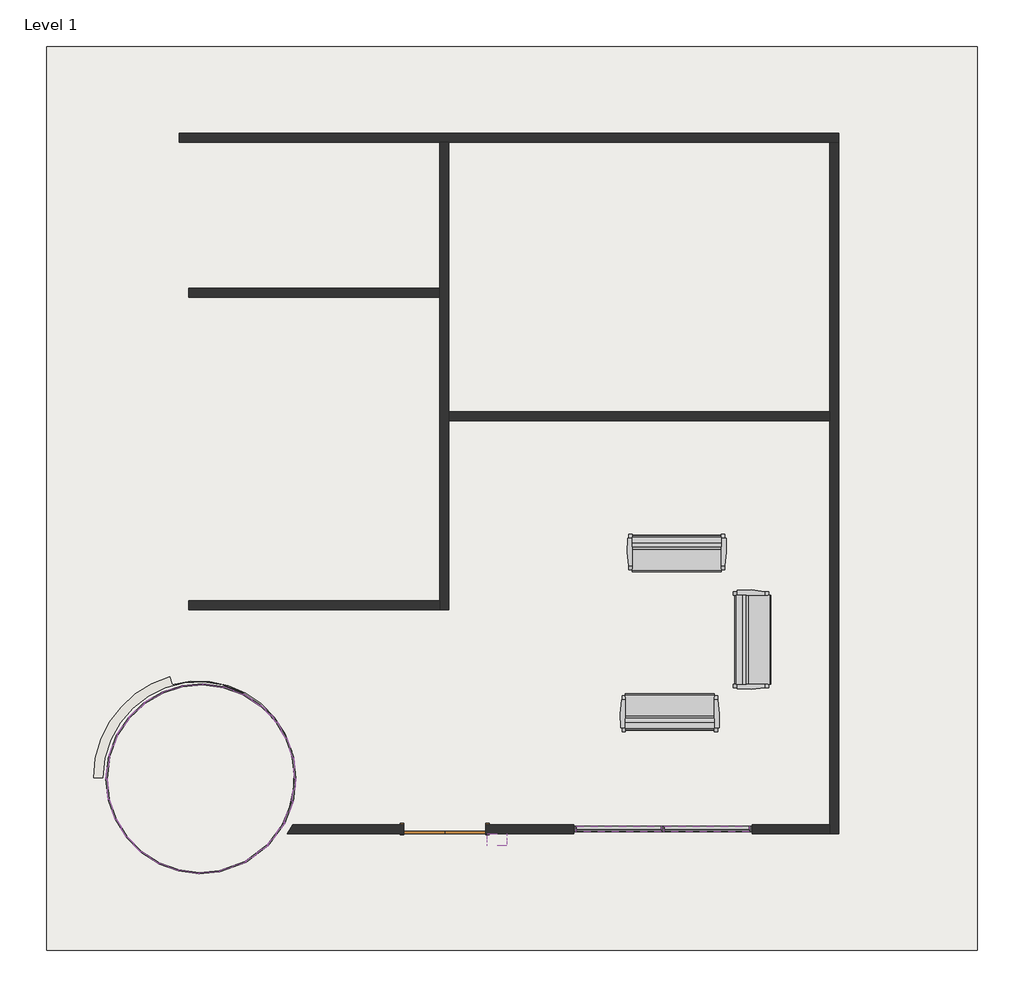
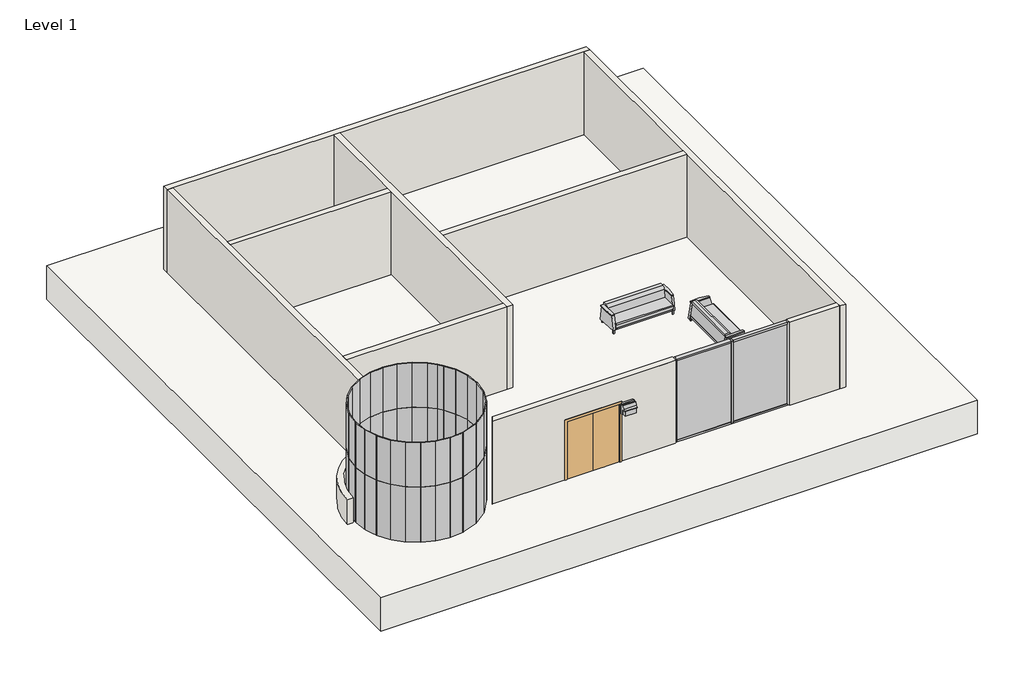
# One storey, incomplete: 58 plates, 11 walls, 7 members, 3 furniture elements, 1 door, 1 light fixture, 1 slab.
"""IFC4 building model written with IfcOpenShell, lengths in millimetres."""

from ifc_helpers import new_model, si_unit, point, frame, frame_2d, origin, origin_with_axes, place, context, project, spatial, polyline, circle_curve, trimmed, segment, composite_curve, outline, extrude, faceted_brep, transform, mapped, element, save
from ifc_brep_helpers import plane_surface, revolved_surface, advanced_brep
from components import door_0b985982, furniture_aff9b2fb, wall_pack_light_exterior_120v_50d39a1a, member_eaba9652, member_3f395ae9, member_7b893d20, system_panel_glazed_c6a8e7fc, system_panel_glazed_f1c144f9, system_panel_glazed_8ed2b2ee, system_panel_glazed_c7815b78, system_panel_glazed_220ba5f3, system_panel_glazed_11fb153e, system_panel_glazed_2f540b85, system_panel_glazed_4848e608, system_panel_glazed_8b35a0ff, system_panel_glazed_87282c25, system_panel_glazed_6d1bb68c, system_panel_glazed_cb3ffd69, system_panel_glazed_404d015f

model = new_model("IFC4")

# Units and contexts
model_context = context("Model", 3, world=origin())
ifc_project = project(units=[si_unit("LENGTHUNIT", "METRE", prefix="MILLI")], contexts=[model_context])

# Site, building, storey
site = spatial("IfcSite", under=ifc_project)
building = spatial("IfcBuilding", under=site)
storey = spatial("IfcBuildingStorey", under=building, Name="Level 1", Elevation=0.0)

# Door
placement = place(None, origin())
door_shape = door_0b985982(model_context)
element("IfcDoor", 1, ObjectType="Door-Double-Flush_Panel : 72\" x 84\"", at=placement, inside=storey, context=model_context, shape_type="MappedRepresentation", body=[
    mapped(door_shape, transform((-7135.1683746, -2219.4937024, 0.0), x_axis=(-1.0, 0.0, 0.0), y_axis=(0.0, -1.0, 0.0), z_axis=(0.0, 0.0, 1.0))),
])

# Furniture
furniture_shape = furniture_aff9b2fb(model_context)
element("IfcFurniture", 2, ObjectType="Sofa-Pensi : 84\"", at=placement, inside=storey, context=model_context, shape_type="MappedRepresentation", body=[
    mapped(furniture_shape, transform((-2244.8524991, 3650.1964615, 0.0), x_axis=(1.0, 0.0, 0.0), y_axis=(0.0, 1.0, 0.0), z_axis=(0.0, 0.0, 1.0))),
])
element("IfcFurniture", 3, ObjectType="Sofa-Pensi : 84\"", at=placement, inside=storey, context=model_context, shape_type="MappedRepresentation", body=[
    mapped(furniture_shape, transform((-12.736413, 1720.492712, 0.0), x_axis=(0.0, 1.0000000000000002, 0.0), y_axis=(-1.0000000000000002, 0.0, 0.0), z_axis=(0.0, 0.0, 1.0))),
])
element("IfcFurniture", 4, ObjectType="Sofa-Pensi : 84\"", at=placement, inside=storey, context=model_context, shape_type="MappedRepresentation", body=[
    mapped(furniture_shape, transform((-1840.0399991, 648.4161336, 0.0), x_axis=(-1.0000000000000004, 0.0, 0.0), y_axis=(0.0, -1.0000000000000004, 0.0), z_axis=(0.0, 0.0, 1.0))),
])

# Light fixture
wall_pack_light_exterior_120v_shape = wall_pack_light_exterior_120v_50d39a1a(model_context)
element("IfcLightFixture", 5, ObjectType="Wall Pack Light - Exterior : 120V", at=placement, inside=storey, context=model_context, shape_type="MappedRepresentation", body=[
    mapped(wall_pack_light_exterior_120v_shape, transform((-5845.0043181, -2219.4937024, -589.106918), x_axis=(-1.0, 0.0, 0.0), y_axis=(0.0, -1.0, 0.0), z_axis=(0.0, 0.0, 1.0))),
])

# Members
member_shape = member_eaba9652(model_context)
element("IfcMember", 6, ObjectType="Rectangular Mullion : 2.5\" x 5\" rectangular", at=placement, inside=storey, context=model_context, shape_type="MappedRepresentation", body=[
    mapped(member_shape, transform((-2277.4073118, -2219.4937024, 0.0), x_axis=(-1.0, 0.0, 0.0), y_axis=(0.0, 1.0, 0.0), z_axis=(0.0, 0.0, -1.0))),
])
member_2_shape = member_3f395ae9(model_context)
element("IfcMember", 7, ObjectType="Rectangular Mullion : 2.5\" x 5\" rectangular", at=placement, inside=storey, context=model_context, shape_type="MappedRepresentation", body=[
    mapped(member_2_shape, transform((-4264.9683746, -2219.4937024, 0.0), x_axis=(-1.0, 0.0, 0.0), y_axis=(0.0, 1.0, 0.0), z_axis=(0.0, 0.0, -1.0))),
])
element("IfcMember", 8, ObjectType="Rectangular Mullion : 2.5\" x 5\" rectangular", at=placement, inside=storey, context=model_context, shape_type="MappedRepresentation", body=[
    mapped(member_2_shape, transform((-289.8462491, -2219.4937024, 3048.0), x_axis=(1.0, 0.0, 0.0), y_axis=(0.0, 1.0, 0.0), z_axis=(0.0, 0.0, 1.0))),
])
member_3_shape = member_7b893d20(model_context)
element("IfcMember", 9, ObjectType="Rectangular Mullion : 2.5\" x 5\" rectangular", at=placement, inside=storey, context=model_context, shape_type="MappedRepresentation", body=[
    mapped(member_3_shape, transform((-4201.4683746, -2219.4937024, 3048.0), x_axis=(0.0, 0.0, 1.0), y_axis=(0.0, 1.0, 0.0), z_axis=(-1.0, 0.0, 0.0))),
])
element("IfcMember", 10, ObjectType="Rectangular Mullion : 2.5\" x 5\" rectangular", at=placement, inside=storey, context=model_context, shape_type="MappedRepresentation", body=[
    mapped(member_3_shape, transform((-2245.6573118, -2219.4937024, 3048.0), x_axis=(0.0, 0.0, 1.0), y_axis=(0.0, 1.0, 0.0), z_axis=(-1.0, 0.0, 0.0))),
])
element("IfcMember", 11, ObjectType="Rectangular Mullion : 2.5\" x 5\" rectangular", at=placement, inside=storey, context=model_context, shape_type="MappedRepresentation", body=[
    mapped(member_3_shape, transform((-353.3462491, -2219.4937024, 0.0), x_axis=(0.0, 0.0, -1.0), y_axis=(0.0, 1.0, 0.0), z_axis=(1.0, 0.0, 0.0))),
])
element("IfcMember", 12, ObjectType="Rectangular Mullion : 2.5\" x 5\" rectangular", at=placement, inside=storey, context=model_context, shape_type="MappedRepresentation", body=[
    mapped(member_3_shape, transform((-2309.1573118, -2219.4937024, 0.0), x_axis=(0.0, 0.0, -1.0), y_axis=(0.0, 1.0, 0.0), z_axis=(1.0, 0.0, 0.0))),
])

# Plates
system_panel_glazed_shape = system_panel_glazed_c6a8e7fc(model_context)
element("IfcPlate", 13, ObjectType="System Panel : Glazed", at=placement, inside=storey, context=model_context, shape_type="MappedRepresentation", body=[
    mapped(system_panel_glazed_shape, transform((-1299.5017804, -2219.4937024, 63.5), x_axis=(-1.0, 0.0, 0.0), y_axis=(0.0, -1.0, 0.0), z_axis=(0.0, 0.0, 1.0))),
])
element("IfcPlate", 14, ObjectType="System Panel : Glazed", at=placement, inside=storey, context=model_context, shape_type="MappedRepresentation", body=[
    mapped(system_panel_glazed_shape, transform((-3255.3128432, -2219.4937024, 63.5), x_axis=(-1.0, 0.0, 0.0), y_axis=(0.0, -1.0, 0.0), z_axis=(0.0, 0.0, 1.0))),
])
system_panel_glazed_2_shape = system_panel_glazed_f1c144f9(model_context)
element("IfcPlate", 15, ObjectType="System Panel : Glazed", at=placement, inside=storey, context=model_context, shape_type="MappedRepresentation", body=[
    mapped(system_panel_glazed_2_shape, transform((-14541.9245022, -346.5978939, 0.0), x_axis=(-0.3551689475306269, -0.9348021281051873, 0.0), y_axis=(0.9348021281051873, -0.3551689475306269, 0.0), z_axis=(0.0, 0.0, 1.0))),
])
element("IfcPlate", 16, ObjectType="System Panel : Glazed", at=placement, inside=storey, context=model_context, shape_type="MappedRepresentation", body=[
    mapped(system_panel_glazed_2_shape, transform((-10582.1178502, -1851.0877948, 0.0), x_axis=(0.35516894753064066, 0.934802128105182, 0.0), y_axis=(-0.934802128105182, 0.35516894753064066, 0.0), z_axis=(0.0, 0.0, 1.0))),
])
element("IfcPlate", 17, ObjectType="System Panel : Glazed", at=placement, inside=storey, context=model_context, shape_type="MappedRepresentation", body=[
    mapped(system_panel_glazed_2_shape, transform((-10459.5232171, -1354.5613954, 0.0), x_axis=(0.12073632210407238, 0.9926846128175765, 0.0), y_axis=(-0.9926846128175765, 0.12073632210407238, 0.0), z_axis=(0.0, 0.0, 1.0))),
])
element("IfcPlate", 18, ObjectType="System Panel : Glazed", at=placement, inside=storey, context=model_context, shape_type="MappedRepresentation", body=[
    mapped(system_panel_glazed_2_shape, transform((-14664.5191354, -843.1242933, 0.0), x_axis=(-0.12073632210406242, -0.9926846128175777, 0.0), y_axis=(0.9926846128175777, -0.12073632210406242, 0.0), z_axis=(0.0, 0.0, 1.0))),
])
system_panel_glazed_3_shape = system_panel_glazed_8ed2b2ee(model_context)
element("IfcPlate", 19, ObjectType="System Panel : Glazed", at=placement, inside=storey, context=model_context, shape_type="MappedRepresentation", body=[
    mapped(system_panel_glazed_3_shape, transform((-11841.3777431, -3082.3793017, 0.0), x_axis=(0.9398911711666007, 0.34147413718036645, 0.0), y_axis=(-0.34147413718036645, 0.9398911711666007, 0.0), z_axis=(0.0, 0.0, 1.0))),
])
element("IfcPlate", 20, ObjectType="System Panel : Glazed", at=placement, inside=storey, context=model_context, shape_type="MappedRepresentation", body=[
    mapped(system_panel_glazed_3_shape, transform((-10858.9635423, -2345.1728692, 0.0), x_axis=(0.5905687200141164, 0.8069873524045393, 0.0), y_axis=(-0.8069873524045393, 0.5905687200141164, 0.0), z_axis=(0.0, 0.0, 1.0))),
])
element("IfcPlate", 21, ObjectType="System Panel : Glazed", at=placement, inside=storey, context=model_context, shape_type="MappedRepresentation", body=[
    mapped(system_panel_glazed_3_shape, transform((-11295.3522982, -2786.8279712, 0.0), x_axis=(0.7998453025525061, 0.6002062078858317, 0.0), y_axis=(-0.6002062078858317, 0.7998453025525061, 0.0), z_axis=(0.0, 0.0, 1.0))),
])
system_panel_glazed_4_shape = system_panel_glazed_c7815b78(model_context)
element("IfcPlate", 22, ObjectType="System Panel : Glazed", at=placement, inside=storey, context=model_context, shape_type="MappedRepresentation", body=[
    mapped(system_panel_glazed_4_shape, transform((-10454.4737362, -864.5204039, 0.0), x_axis=(-0.11050163420416613, 0.993875942378227, 0.0), y_axis=(-0.993875942378227, -0.11050163420416613, 0.0), z_axis=(0.0, 0.0, 1.0))),
])
element("IfcPlate", 23, ObjectType="System Panel : Glazed", at=placement, inside=storey, context=model_context, shape_type="MappedRepresentation", body=[
    mapped(system_panel_glazed_4_shape, transform((-14669.5686163, -1333.1652848, 0.0), x_axis=(0.11050163420415138, -0.9938759423782286, 0.0), y_axis=(0.9938759423782286, 0.11050163420415138, 0.0), z_axis=(0.0, 0.0, 1.0))),
])
element("IfcPlate", 24, ObjectType="System Panel : Glazed", at=placement, inside=storey, context=model_context, shape_type="MappedRepresentation", body=[
    mapped(system_panel_glazed_4_shape, transform((-11410.1424167, 681.5611944, 0.0), x_axis=(-0.8396018558176894, 0.5432022861766066, 0.0), y_axis=(-0.5432022861766066, -0.8396018558176894, 0.0), z_axis=(0.0, 0.0, 1.0))),
])
element("IfcPlate", 25, ObjectType="System Panel : Glazed", at=placement, inside=storey, context=model_context, shape_type="MappedRepresentation", body=[
    mapped(system_panel_glazed_4_shape, transform((-13212.0893695, 919.590846, 0.0), x_axis=(-0.9518517343814786, -0.3065587639506839, 0.0), y_axis=(0.3065587639506839, -0.9518517343814786, 0.0), z_axis=(0.0, 0.0, 1.0))),
])
element("IfcPlate", 26, ObjectType="System Panel : Glazed", at=placement, inside=storey, context=model_context, shape_type="MappedRepresentation", body=[
    mapped(system_panel_glazed_4_shape, transform((-12839.7224363, -3201.1142893, 0.0), x_axis=(0.9913878918151698, -0.1309581916577702, 0.0), y_axis=(0.1309581916577702, 0.9913878918151698, 0.0), z_axis=(0.0, 0.0, 1.0))),
])
element("IfcPlate", 27, ObjectType="System Panel : Glazed", at=placement, inside=storey, context=model_context, shape_type="MappedRepresentation", body=[
    mapped(system_panel_glazed_4_shape, transform((-14365.783041, -2213.7896382, 0.0), x_axis=(0.5257859322352114, -0.8506169252157811, 0.0), y_axis=(0.8506169252157811, 0.5257859322352114, 0.0), z_axis=(0.0, 0.0, 1.0))),
])
element("IfcPlate", 28, ObjectType="System Panel : Glazed", at=placement, inside=storey, context=model_context, shape_type="MappedRepresentation", body=[
    mapped(system_panel_glazed_4_shape, transform((-13713.8999358, -2879.2468831, 0.0), x_axis=(0.8396018558176805, -0.5432022861766201, 0.0), y_axis=(0.5432022861766201, 0.8396018558176805, 0.0), z_axis=(0.0, 0.0, 1.0))),
])
element("IfcPlate", 29, ObjectType="System Panel : Glazed", at=placement, inside=storey, context=model_context, shape_type="MappedRepresentation", body=[
    mapped(system_panel_glazed_4_shape, transform((-14014.4059364, 446.2272921, 0.0), x_axis=(-0.7286232370002992, -0.6849147235263715, 0.0), y_axis=(0.6849147235263715, -0.7286232370002992, 0.0), z_axis=(0.0, 0.0, 1.0))),
])
element("IfcPlate", 30, ObjectType="System Panel : Glazed", at=placement, inside=storey, context=model_context, shape_type="MappedRepresentation", body=[
    mapped(system_panel_glazed_4_shape, transform((-12284.3199161, 1003.4286006, 0.0), x_axis=(-0.9913878918151723, 0.1309581916577514, 0.0), y_axis=(-0.1309581916577514, -0.9913878918151723, 0.0), z_axis=(0.0, 0.0, 1.0))),
])
element("IfcPlate", 31, ObjectType="System Panel : Glazed", at=placement, inside=storey, context=model_context, shape_type="MappedRepresentation", body=[
    mapped(system_panel_glazed_4_shape, transform((-12752.8652893, 1013.0855973, 0.0), x_axis=(-0.9959419324521102, -0.08999815100076568, 0.0), y_axis=(0.08999815100076568, -0.9959419324521102, 0.0), z_axis=(0.0, 0.0, 1.0))),
])
element("IfcPlate", 32, ObjectType="System Panel : Glazed", at=placement, inside=storey, context=model_context, shape_type="MappedRepresentation", body=[
    mapped(system_panel_glazed_4_shape, transform((-11829.3381514, 891.0915272, 0.0), x_axis=(-0.9384120429483949, 0.34551821608913763, 0.0), y_axis=(-0.34551821608913763, -0.9384120429483949, 0.0), z_axis=(0.0, 0.0, 1.0))),
])
element("IfcPlate", 33, ObjectType="System Panel : Glazed", at=placement, inside=storey, context=model_context, shape_type="MappedRepresentation", body=[
    mapped(system_panel_glazed_4_shape, transform((-10557.4115054, -407.3204039, 0.0), x_axis=(-0.3261077326604367, 0.9453326116764772, 0.0), y_axis=(-0.9453326116764772, -0.3261077326604367, 0.0), z_axis=(0.0, 0.0, 1.0))),
])
element("IfcPlate", 34, ObjectType="System Panel : Glazed", at=placement, inside=storey, context=model_context, shape_type="MappedRepresentation", body=[
    mapped(system_panel_glazed_4_shape, transform((-12371.1770631, -3210.771286, 0.0), x_axis=(0.9959419324521115, 0.08999815100075, 0.0), y_axis=(-0.08999815100075, 0.9959419324521115, 0.0), z_axis=(0.0, 0.0, 1.0))),
])
element("IfcPlate", 35, ObjectType="System Panel : Glazed", at=placement, inside=storey, context=model_context, shape_type="MappedRepresentation", body=[
    mapped(system_panel_glazed_4_shape, transform((-13294.7042011, -3088.7772159, 0.0), x_axis=(0.9384120429483891, -0.34551821608915334, 0.0), y_axis=(0.34551821608915334, 0.9384120429483891, 0.0), z_axis=(0.0, 0.0, 1.0))),
])
element("IfcPlate", 36, ObjectType="System Panel : Glazed", at=placement, inside=storey, context=model_context, shape_type="MappedRepresentation", body=[
    mapped(system_panel_glazed_4_shape, transform((-14076.8350959, -2582.7572647, 0.0), x_axis=(0.6997834615185511, -0.7143550286692988, 0.0), y_axis=(0.7143550286692988, 0.6997834615185511, 0.0), z_axis=(0.0, 0.0, 1.0))),
])
element("IfcPlate", 37, ObjectType="System Panel : Glazed", at=placement, inside=storey, context=model_context, shape_type="MappedRepresentation", body=[
    mapped(system_panel_glazed_4_shape, transform((-14566.6308471, -1790.3652848, 0.0), x_axis=(0.32610773266042153, -0.9453326116764824, 0.0), y_axis=(0.9453326116764824, 0.32610773266042153, 0.0), z_axis=(0.0, 0.0, 1.0))),
])
element("IfcPlate", 38, ObjectType="System Panel : Glazed", at=placement, inside=storey, context=model_context, shape_type="MappedRepresentation", body=[
    mapped(system_panel_glazed_4_shape, transform((-14318.3113206, 89.4787227, 0.0), x_axis=(-0.5603879632167612, -0.8282302401396425, 0.0), y_axis=(0.8282302401396425, -0.5603879632167612, 0.0), z_axis=(0.0, 0.0, 1.0))),
])
element("IfcPlate", 39, ObjectType="System Panel : Glazed", at=placement, inside=storey, context=model_context, shape_type="MappedRepresentation", body=[
    mapped(system_panel_glazed_4_shape, transform((-13639.5625299, 727.5108588, 0.0), x_axis=(-0.8612707706620223, -0.508146297441245, 0.0), y_axis=(0.508146297441245, -0.8612707706620223, 0.0), z_axis=(0.0, 0.0, 1.0))),
])
system_panel_glazed_5_shape = system_panel_glazed_220ba5f3(model_context)
element("IfcPlate", 40, ObjectType="System Panel : Glazed", at=placement, inside=storey, context=model_context, shape_type="MappedRepresentation", body=[
    mapped(system_panel_glazed_5_shape, transform((-10742.3305673, -4.7597883, 0.0), x_axis=(-0.5152811917631037, 0.8570211744263939, 0.0), y_axis=(-0.8570211744263939, -0.5152811917631037, 0.0), z_axis=(0.0, 0.0, 1.0))),
])
system_panel_glazed_6_shape = system_panel_glazed_11fb153e(model_context)
element("IfcPlate", 41, ObjectType="System Panel : Glazed", at=placement, inside=storey, context=model_context, shape_type="MappedRepresentation", body=[
    mapped(system_panel_glazed_6_shape, transform((-11098.0043985, 445.2241463, 0.0), x_axis=(-0.7256671855033587, 0.6880458821064435, 0.0), y_axis=(-0.6880458821064435, -0.7256671855033587, 0.0), z_axis=(0.0, 0.0, 1.0))),
])
system_panel_glazed_7_shape = system_panel_glazed_2f540b85(model_context)
element("IfcPlate", 42, ObjectType="System Panel : Glazed", at=placement, inside=storey, context=model_context, shape_type="MappedRepresentation", body=[
    mapped(system_panel_glazed_7_shape, transform((-10917.0903061, 255.9395759, 0.0), x_axis=(-0.6357445726375757, 0.7718995001694627, 0.0), y_axis=(-0.7718995001694627, -0.6357445726375757, 0.0), z_axis=(0.0, 0.0, 1.0))),
])
system_panel_glazed_8_shape = system_panel_glazed_4848e608(model_context)
element("IfcPlate", 43, ObjectType="System Panel : Glazed", at=placement, inside=storey, context=model_context, shape_type="MappedRepresentation", body=[
    mapped(system_panel_glazed_8_shape, transform((-14669.5686163, -1333.1652848, 2032.0), x_axis=(0.11050163420415136, -0.9938759423782286, 0.0), y_axis=(0.9938759423782286, 0.11050163420415136, 0.0), z_axis=(0.0, 0.0, 1.0))),
])
element("IfcPlate", 44, ObjectType="System Panel : Glazed", at=placement, inside=storey, context=model_context, shape_type="MappedRepresentation", body=[
    mapped(system_panel_glazed_8_shape, transform((-14365.783041, -2213.7896382, 2032.0), x_axis=(0.5257859322352114, -0.8506169252157811, 0.0), y_axis=(0.8506169252157811, 0.5257859322352114, 0.0), z_axis=(0.0, 0.0, 1.0))),
])
element("IfcPlate", 45, ObjectType="System Panel : Glazed", at=placement, inside=storey, context=model_context, shape_type="MappedRepresentation", body=[
    mapped(system_panel_glazed_8_shape, transform((-13713.8999358, -2879.2468831, 2032.0), x_axis=(0.8396018558176804, -0.5432022861766203, 0.0), y_axis=(0.5432022861766203, 0.8396018558176804, 0.0), z_axis=(0.0, 0.0, 1.0))),
])
element("IfcPlate", 46, ObjectType="System Panel : Glazed", at=placement, inside=storey, context=model_context, shape_type="MappedRepresentation", body=[
    mapped(system_panel_glazed_8_shape, transform((-12839.7224363, -3201.1142893, 2032.0), x_axis=(0.9913878918151698, -0.1309581916577702, 0.0), y_axis=(0.1309581916577702, 0.9913878918151698, 0.0), z_axis=(0.0, 0.0, 1.0))),
])
element("IfcPlate", 47, ObjectType="System Panel : Glazed", at=placement, inside=storey, context=model_context, shape_type="MappedRepresentation", body=[
    mapped(system_panel_glazed_8_shape, transform((-12371.1770631, -3210.771286, 2032.0), x_axis=(0.9959419324521115, 0.08999815100075, 0.0), y_axis=(-0.08999815100075, 0.9959419324521115, 0.0), z_axis=(0.0, 0.0, 1.0))),
])
element("IfcPlate", 48, ObjectType="System Panel : Glazed", at=placement, inside=storey, context=model_context, shape_type="MappedRepresentation", body=[
    mapped(system_panel_glazed_8_shape, transform((-13294.7042011, -3088.7772159, 2032.0), x_axis=(0.9384120429483891, -0.34551821608915334, 0.0), y_axis=(0.34551821608915334, 0.9384120429483891, 0.0), z_axis=(0.0, 0.0, 1.0))),
])
element("IfcPlate", 49, ObjectType="System Panel : Glazed", at=placement, inside=storey, context=model_context, shape_type="MappedRepresentation", body=[
    mapped(system_panel_glazed_8_shape, transform((-14076.8350959, -2582.7572647, 2032.0), x_axis=(0.6997834615185511, -0.7143550286692988, 0.0), y_axis=(0.7143550286692988, 0.6997834615185511, 0.0), z_axis=(0.0, 0.0, 1.0))),
])
element("IfcPlate", 50, ObjectType="System Panel : Glazed", at=placement, inside=storey, context=model_context, shape_type="MappedRepresentation", body=[
    mapped(system_panel_glazed_8_shape, transform((-14566.6308471, -1790.3652848, 2032.0), x_axis=(0.32610773266042153, -0.9453326116764824, 0.0), y_axis=(0.9453326116764824, 0.32610773266042153, 0.0), z_axis=(0.0, 0.0, 1.0))),
])
element("IfcPlate", 51, ObjectType="System Panel : Glazed", at=placement, inside=storey, context=model_context, shape_type="MappedRepresentation", body=[
    mapped(system_panel_glazed_8_shape, transform((-10454.4737362, -864.5204039, 2032.0), x_axis=(-0.11050163420416614, 0.993875942378227, 0.0), y_axis=(-0.993875942378227, -0.11050163420416614, 0.0), z_axis=(0.0, 0.0, 1.0))),
])
element("IfcPlate", 52, ObjectType="System Panel : Glazed", at=placement, inside=storey, context=model_context, shape_type="MappedRepresentation", body=[
    mapped(system_panel_glazed_8_shape, transform((-10557.4115054, -407.3204039, 2032.0), x_axis=(-0.32610773266043674, 0.9453326116764772, 0.0), y_axis=(-0.9453326116764772, -0.32610773266043674, 0.0), z_axis=(0.0, 0.0, 1.0))),
])
element("IfcPlate", 53, ObjectType="System Panel : Glazed", at=placement, inside=storey, context=model_context, shape_type="MappedRepresentation", body=[
    mapped(system_panel_glazed_8_shape, transform((-11410.1424167, 681.5611944, 2032.0), x_axis=(-0.8396018558176894, 0.5432022861766066, 0.0), y_axis=(-0.5432022861766066, -0.8396018558176894, 0.0), z_axis=(0.0, 0.0, 1.0))),
])
element("IfcPlate", 54, ObjectType="System Panel : Glazed", at=placement, inside=storey, context=model_context, shape_type="MappedRepresentation", body=[
    mapped(system_panel_glazed_8_shape, transform((-11829.3381514, 891.0915272, 2032.0), x_axis=(-0.9384120429483949, 0.34551821608913763, 0.0), y_axis=(-0.34551821608913763, -0.9384120429483949, 0.0), z_axis=(0.0, 0.0, 1.0))),
])
element("IfcPlate", 55, ObjectType="System Panel : Glazed", at=placement, inside=storey, context=model_context, shape_type="MappedRepresentation", body=[
    mapped(system_panel_glazed_8_shape, transform((-12284.3199161, 1003.4286006, 2032.0), x_axis=(-0.9913878918151723, 0.1309581916577514, 0.0), y_axis=(-0.1309581916577514, -0.9913878918151723, 0.0), z_axis=(0.0, 0.0, 1.0))),
])
element("IfcPlate", 56, ObjectType="System Panel : Glazed", at=placement, inside=storey, context=model_context, shape_type="MappedRepresentation", body=[
    mapped(system_panel_glazed_8_shape, transform((-12752.8652893, 1013.0855973, 2032.0), x_axis=(-0.9959419324521102, -0.08999815100076568, 0.0), y_axis=(0.08999815100076568, -0.9959419324521102, 0.0), z_axis=(0.0, 0.0, 1.0))),
])
element("IfcPlate", 57, ObjectType="System Panel : Glazed", at=placement, inside=storey, context=model_context, shape_type="MappedRepresentation", body=[
    mapped(system_panel_glazed_8_shape, transform((-13212.0893695, 919.590846, 2032.0), x_axis=(-0.9518517343814786, -0.3065587639506839, 0.0), y_axis=(0.3065587639506839, -0.9518517343814786, 0.0), z_axis=(0.0, 0.0, 1.0))),
])
element("IfcPlate", 58, ObjectType="System Panel : Glazed", at=placement, inside=storey, context=model_context, shape_type="MappedRepresentation", body=[
    mapped(system_panel_glazed_8_shape, transform((-13639.5625299, 727.5108588, 2032.0), x_axis=(-0.8612707706620223, -0.508146297441245, 0.0), y_axis=(0.508146297441245, -0.8612707706620223, 0.0), z_axis=(0.0, 0.0, 1.0))),
])
element("IfcPlate", 59, ObjectType="System Panel : Glazed", at=placement, inside=storey, context=model_context, shape_type="MappedRepresentation", body=[
    mapped(system_panel_glazed_8_shape, transform((-14014.4059364, 446.2272921, 2032.0), x_axis=(-0.7286232370002992, -0.6849147235263715, 0.0), y_axis=(0.6849147235263715, -0.7286232370002992, 0.0), z_axis=(0.0, 0.0, 1.0))),
])
element("IfcPlate", 60, ObjectType="System Panel : Glazed", at=placement, inside=storey, context=model_context, shape_type="MappedRepresentation", body=[
    mapped(system_panel_glazed_8_shape, transform((-14318.3113206, 89.4787227, 2032.0), x_axis=(-0.5603879632167612, -0.8282302401396425, 0.0), y_axis=(0.8282302401396425, -0.5603879632167612, 0.0), z_axis=(0.0, 0.0, 1.0))),
])
system_panel_glazed_9_shape = system_panel_glazed_8b35a0ff(model_context)
element("IfcPlate", 61, ObjectType="System Panel : Glazed", at=placement, inside=storey, context=model_context, shape_type="MappedRepresentation", body=[
    mapped(system_panel_glazed_9_shape, transform((-10742.3305673, -4.7597883, 2032.0), x_axis=(-0.5152811917631037, 0.8570211744263939, 0.0), y_axis=(-0.8570211744263939, -0.5152811917631037, 0.0), z_axis=(0.0, 0.0, 1.0))),
])
system_panel_glazed_10_shape = system_panel_glazed_87282c25(model_context)
element("IfcPlate", 62, ObjectType="System Panel : Glazed", at=placement, inside=storey, context=model_context, shape_type="MappedRepresentation", body=[
    mapped(system_panel_glazed_10_shape, transform((-10917.0903061, 255.9395759, 2032.0), x_axis=(-0.6357445726375758, 0.7718995001694626, 0.0), y_axis=(-0.7718995001694626, -0.6357445726375758, 0.0), z_axis=(0.0, 0.0, 1.0))),
])
system_panel_glazed_11_shape = system_panel_glazed_6d1bb68c(model_context)
element("IfcPlate", 63, ObjectType="System Panel : Glazed", at=placement, inside=storey, context=model_context, shape_type="MappedRepresentation", body=[
    mapped(system_panel_glazed_11_shape, transform((-11098.0043985, 445.2241463, 2032.0), x_axis=(-0.7256671855033587, 0.6880458821064435, 0.0), y_axis=(-0.6880458821064435, -0.7256671855033587, 0.0), z_axis=(0.0, 0.0, 1.0))),
])
system_panel_glazed_12_shape = system_panel_glazed_cb3ffd69(model_context)
element("IfcPlate", 64, ObjectType="System Panel : Glazed", at=placement, inside=storey, context=model_context, shape_type="MappedRepresentation", body=[
    mapped(system_panel_glazed_12_shape, transform((-10582.1178502, -1851.0877948, 2032.0), x_axis=(0.35516894753064066, 0.934802128105182, 0.0), y_axis=(-0.934802128105182, 0.35516894753064066, 0.0), z_axis=(0.0, 0.0, 1.0))),
])
element("IfcPlate", 65, ObjectType="System Panel : Glazed", at=placement, inside=storey, context=model_context, shape_type="MappedRepresentation", body=[
    mapped(system_panel_glazed_12_shape, transform((-10459.5232171, -1354.5613954, 2032.0), x_axis=(0.12073632210407238, 0.9926846128175765, 0.0), y_axis=(-0.9926846128175765, 0.12073632210407238, 0.0), z_axis=(0.0, 0.0, 1.0))),
])
element("IfcPlate", 66, ObjectType="System Panel : Glazed", at=placement, inside=storey, context=model_context, shape_type="MappedRepresentation", body=[
    mapped(system_panel_glazed_12_shape, transform((-14541.9245022, -346.5978939, 2032.0), x_axis=(-0.3551689475306269, -0.9348021281051873, 0.0), y_axis=(0.9348021281051873, -0.3551689475306269, 0.0), z_axis=(0.0, 0.0, 1.0))),
])
element("IfcPlate", 67, ObjectType="System Panel : Glazed", at=placement, inside=storey, context=model_context, shape_type="MappedRepresentation", body=[
    mapped(system_panel_glazed_12_shape, transform((-14664.5191354, -843.1242933, 2032.0), x_axis=(-0.12073632210406239, -0.9926846128175777, 0.0), y_axis=(0.9926846128175777, -0.12073632210406239, 0.0), z_axis=(0.0, 0.0, 1.0))),
])
system_panel_glazed_13_shape = system_panel_glazed_404d015f(model_context)
element("IfcPlate", 68, ObjectType="System Panel : Glazed", at=placement, inside=storey, context=model_context, shape_type="MappedRepresentation", body=[
    mapped(system_panel_glazed_13_shape, transform((-11841.3777431, -3082.3793017, 2032.0), x_axis=(0.9398911711666007, 0.3414741371803665, 0.0), y_axis=(-0.3414741371803665, 0.9398911711666007, 0.0), z_axis=(0.0, 0.0, 1.0))),
])
element("IfcPlate", 69, ObjectType="System Panel : Glazed", at=placement, inside=storey, context=model_context, shape_type="MappedRepresentation", body=[
    mapped(system_panel_glazed_13_shape, transform((-10858.9635423, -2345.1728692, 2032.0), x_axis=(0.5905687200141164, 0.8069873524045393, 0.0), y_axis=(-0.8069873524045393, 0.5905687200141164, 0.0), z_axis=(0.0, 0.0, 1.0))),
])
element("IfcPlate", 70, ObjectType="System Panel : Glazed", at=placement, inside=storey, context=model_context, shape_type="MappedRepresentation", body=[
    mapped(system_panel_glazed_13_shape, transform((-11295.3522982, -2786.8279712, 2032.0), x_axis=(0.7998453025525061, 0.6002062078858317, 0.0), y_axis=(-0.6002062078858317, 0.7998453025525061, 0.0), z_axis=(0.0, 0.0, 1.0))),
])

# Slab
element("IfcSlab", 71, ObjectType="Generic - 4'", at=placement, inside=storey, context=model_context, shape_type="SweptSolid", body=[
    extrude(outline(polyline([(4727.2589354, 15203.2445399), (4727.2589354, -4913.5554601), (-15999.1410646, -4913.5554601), (-15999.1410646, 15203.2445399), (4727.2589354, 15203.2445399)])), frame((0.0, 0.0, -1219.2), z_axis=(0.0, 0.0, 1.0), x_axis=(1.0, 0.0, 0.0)), (0.0, 0.0, 1.0), 1219.2),
])

# Walls
element("IfcWall", 72, ObjectType="Generic - 8\"", at=placement, inside=storey, context=model_context, shape_type="Brep", body=[
    faceted_brep([(-13040.6462491, 13071.3062976, 0.0), (-12837.4462491, 13071.3062976, 0.0), (-7249.4462491, 13071.3062976, 0.0), (-7046.2462491, 13071.3062976, 0.0), (1437.3537509, 13071.3062976, 0.0), (1640.5537509, 13071.3062976, 0.0), (1640.5537509, 13071.3062976, 3048.0), (1437.3537509, 13071.3062976, 3048.0), (-7046.2462491, 13071.3062976, 3048.0), (-7249.4462491, 13071.3062976, 3048.0), (-12837.4462491, 13071.3062976, 3048.0), (-13040.6462491, 13071.3062976, 3048.0), (-13040.6462491, 13274.5062976, 0.0), (-13040.6462491, 13274.5062976, 3048.0), (1640.5537509, 13274.5062976, 3048.0), (1640.5537509, 13274.5062976, 0.0)], [[[0, 1, 2, 3, 4, 5, 6, 7, 8, 9, 10, 11]], [[12, 13, 14, 15]], [[5, 4, 3, 2, 1, 0, 12, 15]], [[11, 10, 9, 8, 7, 6, 14, 13]], [[6, 5, 15, 14]], [[0, 11, 13, 12]]]),
])
element("IfcWall", 73, ObjectType="Generic - 8\"", at=placement, inside=storey, context=model_context, shape_type="Brep", body=[
    faceted_brep([(1437.3537509, 13071.3062976, 0.0), (1437.3537509, 7076.9062976, 0.0), (1437.3537509, 6873.7062976, 0.0), (1437.3537509, -2117.8937024, 0.0), (1437.3537509, -2321.0937024, 0.0), (1437.3537509, -2321.0937024, 3048.0), (1437.3537509, -2117.8937024, 3048.0), (1437.3537509, 6873.7062976, 3048.0), (1437.3537509, 7076.9062976, 3048.0), (1437.3537509, 13071.3062976, 3048.0), (1640.5537509, 13071.3062976, 0.0), (1640.5537509, 13071.3062976, 3048.0), (1640.5537509, -2321.0937024, 3048.0), (1640.5537509, -2321.0937024, 0.0)], [[[0, 1, 2, 3, 4, 5, 6, 7, 8, 9]], [[10, 11, 12, 13]], [[4, 3, 2, 1, 0, 10, 13]], [[9, 8, 7, 6, 5, 12, 11]], [[0, 9, 11, 10]], [[5, 4, 13, 12]]]),
])
element("IfcWall", 74, ObjectType="Generic - 8\"", at=placement, inside=storey, context=model_context, shape_type="AdvancedBrep", body=[
    advanced_brep(
    [(-13040.6462491, 13071.3062976, 0.0), (-13040.6462491, 1241.1937063, 0.0), (-13040.6462491, 1241.1937063, 3048.0), (-13040.6462491, 13071.3062976, 3048.0), (-12837.4462491, 13071.3062976, 0.0), (-12837.4462491, 13071.3062976, 3048.0), (-12837.4462491, 9820.1062976, 3048.0), (-12837.4462491, 9616.9062976, 3048.0), (-12837.4462491, 2862.698962, 3048.0), (-12837.4462491, 2659.498962, 3048.0), (-12837.4462491, 1269.6553935, 3048.0), (-12837.4462491, 1269.6553935, 0.0), (-12837.4462491, 2659.498962, 0.0), (-12837.4462491, 2862.698962, 0.0), (-12837.4462491, 9616.9062976, 0.0), (-12837.4462491, 9820.1062976, 0.0)],
    [
        (0, 1),
        (1, 2),
        (2, 3),
        (3, 0),
        (4, 5),
        (5, 6),
        (6, 7),
        (7, 8),
        (8, 9),
        (9, 10),
        (10, 11),
        (11, 12),
        (12, 13),
        (13, 14),
        (14, 15),
        (15, 4),
        (0, 4),
        (11, 1, circle_curve(frame((-12612.6150686, -1075.1054509, 0.0), z_axis=(0.0, 0.0, 1.0), x_axis=(1.0, 0.0, 0.0)), 2355.5153315)),
        (2, 10, circle_curve(frame((-12612.6150686, -1075.1054509, 3048.0), z_axis=(0.0, 0.0, -1.0), x_axis=(1.0, 0.0, 0.0)), 2355.5153315)),
        (5, 3),
    ],
    [
        plane_surface(frame((-13040.6462491, 16068.5062976, 0.0), z_axis=(-1.0, 0.0, 0.0), x_axis=(0.0, -1.0, 0.0))),
        plane_surface(frame((-12837.4462491, 16068.5062976, 0.0), z_axis=(1.0, 0.0, 0.0), x_axis=(0.0, 1.0, 0.0))),
        plane_surface(frame((-13040.6462491, 13172.9062976, 0.0), z_axis=(0.0, 0.0, -1.0), x_axis=(1.0, 0.0, 0.0))),
        plane_surface(frame((-13040.6462491, 1155.046339, 3048.0), z_axis=(0.0, 0.0, 1.0), x_axis=(1.0, 0.0, 0.0))),
        plane_surface(frame((-16139.4462491, 13071.3062976, 0.0), z_axis=(0.0, 1.0, 0.0), x_axis=(1.0, 0.0, 0.0))),
        revolved_surface(polyline([(-10257.099737100001, -1075.1054509, 3048.0), (-10257.099737100001, -1075.1054509, 0.0)]), (-12612.6150686, -1075.1054509, 0.0), (0.0, 0.0, 1.0)),
    ],
    [
        (0, [[1, 2, 3, 4]]),
        (1, [[5, 6, 7, 8, 9, 10, 11, 12, 13, 14, 15, 16]]),
        (2, [[-1, 17, -16, -15, -14, -13, -12, 18]]),
        (3, [[-3, 19, -10, -9, -8, -7, -6, 20]]),
        (4, [[-4, -20, -5, -17]]),
        (5, [[-18, -11, -19, -2]]),
    ],
),
])
element("IfcWall", 75, ObjectType="Generic - 8\"", at=placement, inside=storey, context=model_context, shape_type="AdvancedBrep", body=[
    advanced_brep(
    [(-4264.9683746, -2321.0937024, 0.0), (-4264.9683746, -2321.0937024, 3048.0), (-10635.7115512, -2321.0937024, 3048.0), (-10635.7115512, -2321.0937024, 0.0), (-8049.5683746, -2321.0937024, 0.0), (-8049.5683746, -2321.0937024, 2133.6), (-6220.7683746, -2321.0937024, 2133.6), (-6220.7683746, -2321.0937024, 0.0), (-4264.9683746, -2117.8937024, 3048.0), (-4264.9683746, -2117.8937024, 0.0), (-6220.7683746, -2117.8937024, 0.0), (-6220.7683746, -2117.8937024, 2133.6), (-8049.5683746, -2117.8937024, 2133.6), (-8049.5683746, -2117.8937024, 0.0), (-10521.3888966, -2117.8937024, 0.0), (-10521.3888966, -2117.8937024, 3048.0)],
    [
        (0, 1),
        (1, 2),
        (2, 3),
        (3, 4),
        (4, 5),
        (5, 6),
        (6, 7),
        (7, 0),
        (8, 9),
        (9, 10),
        (10, 11),
        (11, 12),
        (12, 13),
        (13, 14),
        (14, 15),
        (15, 8),
        (9, 0),
        (7, 10),
        (3, 14, circle_curve(frame((-12612.6150686, -1075.1054509, 0.0), z_axis=(0.0, 0.0, 1.0), x_axis=(1.0, 0.0, 0.0)), 2336.8)),
        (13, 4),
        (8, 1),
        (15, 2, circle_curve(frame((-12612.6150686, -1075.1054509, 3048.0), z_axis=(0.0, 0.0, -1.0), x_axis=(1.0, 0.0, 0.0)), 2336.8)),
        (12, 5),
        (11, 6),
    ],
    [
        plane_surface(frame((-9281.4462491, -2321.0937024, 0.0), z_axis=(0.0, -1.0, 0.0), x_axis=(1.0, 0.0, 0.0))),
        plane_surface(frame((-9281.4462491, -2117.8937024, 0.0), z_axis=(0.0, 1.0, 0.0), x_axis=(-1.0, 0.0, 0.0))),
        plane_surface(frame((-10746.4246863, -2321.0937024, 0.0), z_axis=(0.0, 0.0, -1.0), x_axis=(0.0, 1.0, 0.0))),
        plane_surface(frame((-4264.9683746, -2321.0937024, 0.0), z_axis=(1.0, 0.0, 0.0), x_axis=(0.0, 1.0, 0.0))),
        plane_surface(frame((-4264.9683746, -2321.0937024, 3048.0), z_axis=(0.0, 0.0, 1.0), x_axis=(0.0, 1.0, 0.0))),
        revolved_surface(polyline([(-10275.8150686, -1075.1054509, 3048.0), (-10275.8150686, -1075.1054509, 0.0)]), (-12612.6150686, -1075.1054509, 0.0), (0.0, 0.0, 1.0)),
        plane_surface(frame((-8049.5683746, -593.8937024, 0.0), z_axis=(1.0, 0.0, 0.0), x_axis=(0.0, -1.0, 0.0))),
        plane_surface(frame((-8049.5683746, -593.8937024, 2133.6), z_axis=(0.0, 0.0, -1.0), x_axis=(0.0, -1.0, 0.0))),
        plane_surface(frame((-6220.7683746, -593.8937024, 2133.6), z_axis=(-1.0, 0.0, 0.0), x_axis=(0.0, -1.0, 0.0))),
    ],
    [
        (0, [[1, 2, 3, 4, 5, 6, 7, 8]]),
        (1, [[9, 10, 11, 12, 13, 14, 15, 16]]),
        (2, [[17, -8, 18, -10]]),
        (2, [[19, -14, 20, -4]]),
        (3, [[-1, -17, -9, 21]]),
        (4, [[-2, -21, -16, 22]]),
        (5, [[-3, -22, -15, -19]]),
        (6, [[23, -5, -20, -13]]),
        (7, [[-23, -12, 24, -6]]),
        (8, [[-24, -11, -18, -7]]),
    ],
),
])
element("IfcWall", 76, ObjectType="Generic - 8\"", at=placement, inside=storey, context=model_context, shape_type="Brep", body=[
    faceted_brep([(-7249.4462491, 13071.3062976, 0.0), (-7249.4462491, 9820.1062976, 0.0), (-7249.4462491, 9616.9062976, 0.0), (-7249.4462491, 2862.698962, 0.0), (-7249.4462491, 2659.498962, 0.0), (-7249.4462491, 2659.498962, 3048.0), (-7249.4462491, 2862.698962, 3048.0), (-7249.4462491, 9616.9062976, 3048.0), (-7249.4462491, 9820.1062976, 3048.0), (-7249.4462491, 13071.3062976, 3048.0), (-7046.2462491, 13071.3062976, 0.0), (-7046.2462491, 13071.3062976, 3048.0), (-7046.2462491, 7076.9062976, 3048.0), (-7046.2462491, 6873.7062976, 3048.0), (-7046.2462491, 2659.498962, 3048.0), (-7046.2462491, 2659.498962, 0.0), (-7046.2462491, 6873.7062976, 0.0), (-7046.2462491, 7076.9062976, 0.0)], [[[0, 1, 2, 3, 4, 5, 6, 7, 8, 9]], [[10, 11, 12, 13, 14, 15, 16, 17]], [[4, 3, 2, 1, 0, 10, 17, 16, 15]], [[9, 8, 7, 6, 5, 14, 13, 12, 11]], [[0, 9, 11, 10]], [[5, 4, 15, 14]]]),
])
element("IfcWall", 77, ObjectType="Generic - 8\"", at=placement, inside=storey, context=model_context, shape_type="SweptSolid", body=[
    extrude(outline(polyline([(1437.3537509, 6873.7062976), (-7046.2462491, 6873.7062976), (-7046.2462491, 7076.9062976), (1437.3537509, 7076.9062976), (1437.3537509, 6873.7062976)])), origin_with_axes(), (0.0, 0.0, 1.0), 3048.0),
])
element("IfcWall", 78, ObjectType="Generic - 8\"", at=placement, inside=storey, context=model_context, shape_type="SweptSolid", body=[
    extrude(outline(polyline([(-12837.4462491, 9820.1062976), (-7249.4462491, 9820.1062976), (-7249.4462491, 9616.9062976), (-12837.4462491, 9616.9062976), (-12837.4462491, 9820.1062976)])), origin_with_axes(), (0.0, 0.0, 1.0), 3048.0),
])
element("IfcWall", 79, ObjectType="Generic - 8\"", at=placement, inside=storey, context=model_context, shape_type="SweptSolid", body=[
    extrude(outline(polyline([(-12837.4462491, 2862.698962), (-7249.4462491, 2862.698962), (-7249.4462491, 2659.498962), (-12837.4462491, 2659.498962), (-12837.4462491, 2862.698962)])), origin_with_axes(), (0.0, 0.0, 1.0), 3048.0),
])
element("IfcWall", 80, ObjectType="Generic - 8\"", at=placement, inside=storey, context=model_context, shape_type="SweptSolid", body=[
    extrude(outline(composite_curve([segment(trimmed(circle_curve(frame_2d((-12612.6150686, -1075.1054509)), 2133.6), [point((-10751.2065636, -2117.8937024))], [point((-14746.2150686, -1075.1054509))], True, "CARTESIAN"), True, "CONTINUOUS"), segment(polyline([(-14746.2150686, -1075.1054509), (-14949.4150686, -1075.1054509)]), True, "CONTINUOUS"), segment(trimmed(circle_curve(frame_2d((-12612.6150686, -1075.1054509)), 2336.8), [point((-14949.4150686, -1075.1054509))], [point((-13255.6933282, 1171.4662912))], False, "CARTESIAN"), True, "CONTINUOUS"), segment(polyline([(-13255.6933282, 1171.4662912), (-13204.9238659, 994.1049238)]), True, "CONTINUOUS"), segment(trimmed(circle_curve(frame_2d((-12612.6150686, -1075.1054509)), 2152.3153315), [point((-13204.9238659, 994.1049238))], [point((-10729.7837037, -2117.8937024))], False, "CARTESIAN"), True, "CONTINUOUS"), segment(polyline([(-10729.7837037, -2117.8937024), (-10751.2065636, -2117.8937024)]), True, "CONTINUOUS")], self_intersect=False)), origin_with_axes(), (0.0, 0.0, 1.0), 914.4),
])
element("IfcWall", 81, ObjectType="Generic - 8\"", at=placement, inside=storey, context=model_context, shape_type="SweptSolid", body=[
    extrude(outline(polyline([(-4812.8723668, -2321.0937024), (-4812.8723668, -2117.8937024), (-4264.9683746, -2117.8937024), (-4264.9683746, -2321.0937024), (-4812.8723668, -2321.0937024)])), origin_with_axes(), (0.0, 0.0, 1.0), 3048.0),
    extrude(outline(polyline([(1437.3537509, -2117.8937024), (1437.3537509, -2321.0937024), (-289.8462491, -2321.0937024), (-289.8462491, -2117.8937024), (1437.3537509, -2117.8937024)])), origin_with_axes(), (0.0, 0.0, 1.0), 3048.0),
])
element("IfcWall", 82, ObjectType="Generic - 8\" - Filled", at=placement, inside=storey, context=model_context, shape_type="SweptSolid", body=[
    extrude(outline(polyline([(-289.8462491, -2117.8937024), (1437.3537509, -2117.8937024), (1437.3537509, -2321.0937024), (-289.8462491, -2321.0937024), (-289.8462491, -2117.8937024)])), origin_with_axes(), (0.0, 0.0, 1.0), 3048.0),
])

save(model, "model.ifc")

# Revit data of these elements
# Type "Door-Double-Flush_Panel : 72\" x 84\""
#   Type Mark = "9"
#   Construction Type Id = "DOOR"
#   Assembly Code = "C1020"
#   Analytic Construction = "Wooden"
#   Thickness = 0' - 2"
#   Thermal Resistance (R) = 2.5876 (h·ft²·°F)/BTU
#   Swing Angle [instance default] = 90.00°
#   Panel Width = 3' - 0"
#   Heat Transfer Coefficient (U) = 0.3865 BTU/(h·ft²·°F)
#   Height = 7' - 0"
#   Trim Projection Ext = 0' - 1"
#   Trim Projection Int = 0' - 1"
#   Trim Width = 0' - 3"
#   Width = 6' - 0"
#   Define Thermal Properties by = 1
#   Panel Material = Earth
#   Trim Material = Paint - Sienna
#   Visual Light Transmittance = 0
#   Solar Heat Gain Coefficient = 0
#   Function = (empty or 0)
#   Wall Closure = (empty or 0)
# Type "Sofa-Pensi : 84\""
#   Assembly Code = "E2020200"
#   Length = 7' - 0"
#   Frame Material = Cherry
#   Seat Material = Linen, Beige
#   Feet Material = Steel, Chrome Plated
#   Default Elevation = 0
# Type "Wall Pack Light - Exterior : 120V"
#   Assembly Code = "D5020230"
#   Wattage = 70 W
#   built-in parameter 1150110 = 1 (stored number, unit not read)
#   built-in parameter 1114217 = 1 (stored number, unit not read)
#   built-in parameter 1150109 = 1 (stored number, unit not read)
#   built-in parameter 1150113 = 1 (stored number, unit not read)
#   built-in parameter 1150115 = 1 (stored number, unit not read)
#   built-in parameter 1150105 = 437.668 (stored number, unit not read)
#   Light Source Symbol Size = 2' - 0"
#   built-in parameter 1150112 = 1 (stored number, unit not read)
#   built-in parameter 1150114 = 1 (stored number, unit not read)
#   built-in parameter 1150107 = 4000 (stored number, unit not read)
#   built-in parameter 1150106 = 4.37668 (stored number, unit not read)
#   built-in parameter 1150104 = 7.29939 (stored number, unit not read)
#   Ballast Voltage = 120 V
#   built-in parameter 1114218 = 1 (stored number, unit not read)
#   built-in parameter 1150133 = 10 (stored number, unit not read)
#   Lumens = 5499.9 lm
#   Mounting Height = 9' - 0"
#   Apparent Load = 70 VA
#   built-in parameter 1150134 = 12
#   built-in parameter 1150137 = 1
#   Color Filter = 16777215
#   Ballast Number of Poles = 1
#   Wall Mount Material = Metal - Paint Finish - Dark Grey, Matte
#   Shade Material = Glass
#   Load Classification = Lighting - Exterior
#   Dimming Lamp Color Temperature Shift = (empty or 0)
#   Default Elevation = 0
# Type "Rectangular Mullion : 2.5\" x 5\" rectangular"
#   built-in parameter 1007304 = 0.416667 (stored number, unit not read)
#   built-in parameter 1007301 = 0.104167 (stored number, unit not read)
#   built-in parameter 1007300 = 0.104167 (stored number, unit not read)
# Type "System Panel : Glazed"
#   Construction Type Id = "GSP4R"
#   Analytic Construction = "1/8 in Pilkington single glazing"
#   Visual Light Transmittance = 0.9
#   Solar Heat Gain Coefficient = 0.86
#   Heat Transfer Coefficient (U) = 1.18115 BTU/(h·ft²·°F)
# Type "Generic - 4'"
#   Assembly Code = "B1010"
#   Function = 0
#   Layers, outside or top first: 4' - 0" no material (function 1)
# Type "Generic - 8\""
#   Assembly Code = "B2010"
#   Layers, outside or top first: 0' - 8" no material (function 1)
# Type "Generic - 8\" - Filled"
#   Assembly Code = "B2010"
#   Layers, outside or top first: 0' - 8" no material (function 1)
# Element 1 (IfcDoor, "Door-Double-Flush_Panel : 72\" x 84\"")
#   Swing Angle = 90.00°
#   Phase Created = New Construction
#   Materials on its faces: "Paint - Sienna", "Earth"
# Elements 2, 3, 4 (IfcFurniture, "Sofa-Pensi : 84\"")
#   Phase Created = New Construction
#   Materials on its faces: "Cherry", "Linen, Beige", "Steel, Chrome Plated"
# Element 5 (IfcLightFixture, "Wall Pack Light - Exterior : 120V")
#   Mark = "1"
#   Phase Created = New Construction
#   Materials on its faces: "Metal - Paint Finish - Dark Grey, Matte", "Glass"
# Elements 6, 7, 8, 9, 10, 11, 12 (IfcMember, "Rectangular Mullion : 2.5\" x 5\" rectangular")
#   Phase Created = New Construction
#   Materials on its faces: "Iron, Ductile"
# Elements 13, 14, 15, 16, 17, 18, 19, 20, 21, 22, 23, 24, 25, 26, 27, 28, 29, 30, 31, 32, 33, 34, 35, 36, 37, 38, 39, 40, 41, 42, 43, 44, 45, 46, 47, 48, 49, 50, 51, 52, 53, 54, 55, 56, 57, 58, 59, 60, 61, 62, 63, 64, 65, 66, 67, 68, 69, 70 (IfcPlate, "System Panel : Glazed")
#   Phase Created = New Construction
#   Materials on its faces: "Glass"
# Element 71 (IfcSlab, "Generic - 4'")
#   Height Offset From Level = 0' - 0"
#   Phase Created = New Construction
#   Materials on its faces: "Default Floor"
# Elements 72, 73, 74, 75, 76, 77, 78, 79, 81 (IfcWall, "Generic - 8\"")
#   Top Offset = 0' - 0"
#   Base Offset = 0' - 0"
#   Unconnected Height = 10' - 0"
#   wall height = 10' - 0"
#   Phase Created = New Construction
#   Base Constraint = Level 1
#   Materials on its faces: "Default Wall"
# Element 80 (IfcWall, "Generic - 8\"")
#   Top Offset = 0' - 0"
#   Base Offset = 0' - 0"
#   Unconnected Height = 3' - 0"
#   wall height = 3' - 0"
#   Phase Created = New Construction
#   Materials on its faces: "Default Wall"
# Element 82 (IfcWall, "Generic - 8\" - Filled")
#   Top Offset = 0' - 0"
#   Base Offset = 0' - 0"
#   Unconnected Height = 10' - 0"
#   wall height = 10' - 0"
#   Phase Created = New Construction
#   Base Constraint = Level 1
#   Materials on its faces: "Default Wall"
# Materials
#   "Earth": class "Generic", colour RGB 97 75 62, transparency 0, Description = "Soil", Cost = 0
#   "Paint - Sienna": colour RGB 118 70 51, transparency 0, Cost = 0
#   "Cherry": class "Wood", colour RGB 226 177 128, transparency 0, Description = "Prunus Serotina", Cost = 0
#   "Linen, Beige": class "Textile", colour RGB 249 239 230, transparency 0, Description = "Linen, beige", Cost = 0
#   "Steel, Chrome Plated": class "Metal", colour RGB 17 17 17, transparency 0, Description = "Chromiuim plated steel", Cost = 0
#   "Metal - Paint Finish - Dark Grey, Matte": class "Paint", colour RGB 98 98 98, transparency 0
#   "Glass": class "Glass", colour RGB 0 128 192, transparency 0.75, Description = "Soda Lime Glass", Cost = 0
#   "Iron, Ductile": class "Metal", colour RGB 0 0 0, transparency 0, Description = "Ductile cast iron", Cost = 0
#   "Default Floor": colour RGB 128 128 128, transparency 0
#   "Default Wall": colour RGB 128 128 128, transparency 0
